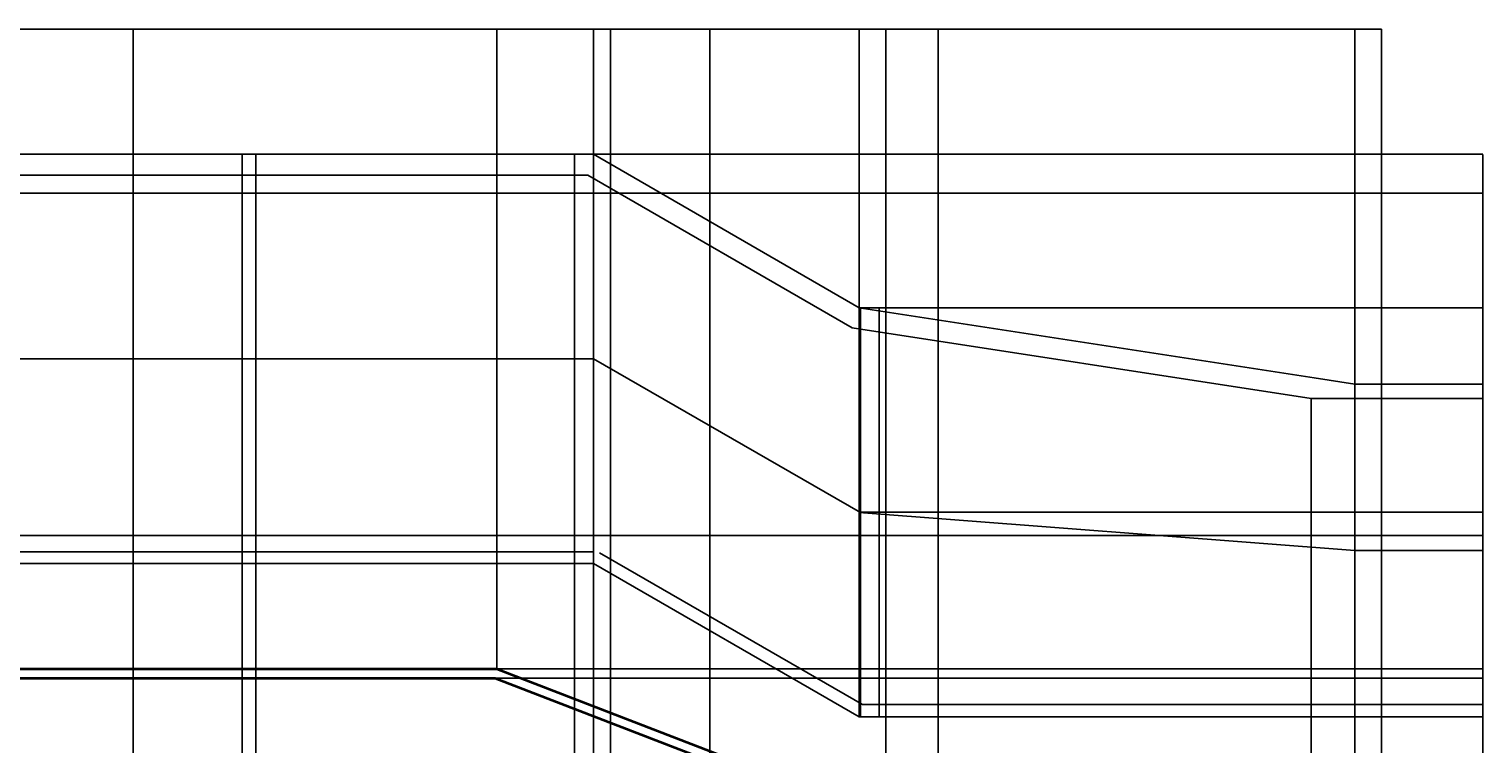
# Model space of a CAD drawing. Units: millimetres. Extents: x 2845 to 7170, y 3531 to 6858.
# Tile 3 of 3: x 4328 to 7170, y 5460 to 6858. Entities that reach past the tile are written whole.
import ezdxf

# ---------------------------------------------------------------- set-up
doc = ezdxf.new("R2010")
doc.units = ezdxf.units.MM
for name, color, linetype, lineweight in [('A-ANNO-DIMS', 2, 'Continuous', 18), ('A-FURN-CTOP', 6, 'Continuous', 35), ('A-FURN-UPPR', 4, 'Continuous', 25)]:
    doc.layers.add(name, color=color, linetype=linetype, lineweight=lineweight)
doc.styles.get("Standard").update_dxf_attribs({"font": 'arial.ttf'})
doc.dimstyles.get("Standard").update_dxf_attribs({"dimtxt": 0.18, "dimasz": 0.18, "dimexe": 0.18, "dimexo": 0.0625, "dimgap": 0.09, "dimtad": 0, "dimtih": 1, "dimtoh": 1, "dimdec": 4, "dimzin": 0, "dimdsep": 46, "dimtxsty": 'Standard', "dimcen": 0.09, "dimadec": 0, "dimazin": 0, "dimtfac": 1, "dimtdec": 4, "dimtofl": 0, "dimtmove": 0, "dimatfit": 3, "dimfxl": 1, "dimtolj": 1, "dimtzin": 0, "dimarcsym": 0})

# ---------------------------------------------------------------- blocks, each defined once
blk = doc.blocks.new('*D1')
at = {"layer": 'A-ANNO-DIMS', "color": 0, "lineweight": -2, "transparency": 16777216}
for p, q in [((3042.6, 6659.7), (2844.7, 6659.7)), ((2844.9, 6659.5), (2844.9, 5194.4)), ((2844.9, 3728.9), (2844.9, 5194)), ((6608, 3728.7), (2844.7, 3728.7))]:
    blk.add_line(p, q, dxfattribs=at)
at = {"layer": 'A-ANNO-DIMS', "color": 0, "transparency": 16777216}
for points in [[(2844.9, 6659.5), (2844.9, 6659.5), (2844.9, 6659.7)], [(2844.9, 3728.9), (2844.9, 3728.9), (2844.9, 3728.7)]]:
    blk.add_solid(points, dxfattribs=at)
at = {"layer": 'Defpoints', "color": 0, "transparency": 16777216}
for p in [(2844.9, 6659.7), (3042.7, 6659.7), (6608.1, 3728.7)]:
    blk.add_point(p, dxfattribs=at)
at = {"layer": 'A-ANNO-DIMS', "color": 0, "transparency": 16777216, "insert": (2844.9, 5194.2), "char_height": 0.18, "attachment_point": 5}
blk.add_mtext('\\A1;2931', dxfattribs=at)
blk = doc.blocks.new('*D2')
at = {"layer": 'A-ANNO-DIMS', "color": 0, "lineweight": -2, "transparency": 16777216}
for p, q in [((3042.7, 6659.8), (3042.7, 6857.7)), ((3042.8, 6857.5), (5006.9, 6857.5)), ((6971.9, 6857.5), (5007.8, 6857.5)), ((6972.1, 4944.1), (6972.1, 6857.7))]:
    blk.add_line(p, q, dxfattribs=at)
at = {"layer": 'A-ANNO-DIMS', "color": 0, "transparency": 16777216}
for points in [[(3042.8, 6857.5), (3042.8, 6857.4), (3042.7, 6857.5)], [(6971.9, 6857.5), (6971.9, 6857.4), (6972.1, 6857.5)]]:
    blk.add_solid(points, dxfattribs=at)
at = {"layer": 'Defpoints', "color": 0, "transparency": 16777216}
for p in [(6972.1, 6857.5), (3042.7, 6659.7), (6972.1, 4944.1)]:
    blk.add_point(p, dxfattribs=at)
at = {"layer": 'A-ANNO-DIMS', "color": 0, "transparency": 16777216, "insert": (5007.4, 6857.5), "char_height": 0.18, "attachment_point": 5}
blk.add_mtext('\\A1;3929.4', dxfattribs=at)
blk = doc.blocks.new('*D6')
at = {"layer": 'A-ANNO-DIMS', "color": 0, "lineweight": -2, "transparency": 16777216}
for p, q in [((4121.4, 6537), (4121.4, 6857.7)), ((4121.6, 6857.5), (4325.9, 6857.5)), ((4531.1, 6857.5), (4326.7, 6857.5)), ((4531.3, 6612.8), (4531.3, 6857.7))]:
    blk.add_line(p, q, dxfattribs=at)
at = {"layer": 'A-ANNO-DIMS', "color": 0, "transparency": 16777216}
for points in [[(4121.6, 6857.5), (4121.6, 6857.4), (4121.4, 6857.5)], [(4531.1, 6857.5), (4531.1, 6857.4), (4531.3, 6857.5)]]:
    blk.add_solid(points, dxfattribs=at)
at = {"layer": 'Defpoints', "color": 0, "transparency": 16777216}
for p in [(4531.3, 6857.5), (4531.3, 6612.8), (4121.4, 6537)]:
    blk.add_point(p, dxfattribs=at)
at = {"layer": 'A-ANNO-DIMS', "color": 0, "transparency": 16777216, "insert": (4326.3, 6857.5), "char_height": 0.18, "attachment_point": 5}
blk.add_mtext('\\A1;409.9', dxfattribs=at)
blk = doc.blocks.new('*D7')
at = {"layer": 'A-ANNO-DIMS', "color": 0, "lineweight": -2, "transparency": 16777216}
for p, q in [((4531.3, 6612.8), (4531.3, 6857.7)), ((4531.4, 6857.5), (4981, 6857.5)), ((5431.1, 6857.5), (4981.6, 6857.5)), ((5431.3, 6612.8), (5431.3, 6857.7))]:
    blk.add_line(p, q, dxfattribs=at)
at = {"layer": 'A-ANNO-DIMS', "color": 0, "transparency": 16777216}
for points in [[(4531.4, 6857.5), (4531.4, 6857.4), (4531.3, 6857.5)], [(5431.1, 6857.5), (5431.1, 6857.4), (5431.3, 6857.5)]]:
    blk.add_solid(points, dxfattribs=at)
at = {"layer": 'Defpoints', "color": 0, "transparency": 16777216}
for p in [(5431.3, 6857.5), (4531.3, 6612.8), (5431.3, 6612.8)]:
    blk.add_point(p, dxfattribs=at)
at = {"layer": 'A-ANNO-DIMS', "color": 0, "transparency": 16777216, "insert": (4981.3, 6857.5), "char_height": 0.18, "attachment_point": 5}
blk.add_mtext('\\A1;900', dxfattribs=at)
blk = doc.blocks.new('*D8')
at = {"layer": 'A-ANNO-DIMS', "color": 0, "lineweight": -2, "transparency": 16777216}
for p, q in [((5431.3, 6612.8), (5431.3, 6857.7)), ((5431.4, 6857.5), (5690.7, 6857.5)), ((5950.7, 6857.5), (5691.5, 6857.5)), ((5950.9, 6312.8), (5950.9, 6857.7))]:
    blk.add_line(p, q, dxfattribs=at)
at = {"layer": 'A-ANNO-DIMS', "color": 0, "transparency": 16777216}
for points in [[(5431.4, 6857.5), (5431.4, 6857.4), (5431.3, 6857.5)], [(5950.7, 6857.5), (5950.7, 6857.4), (5950.9, 6857.5)]]:
    blk.add_solid(points, dxfattribs=at)
at = {"layer": 'Defpoints', "color": 0, "transparency": 16777216}
for p in [(5950.9, 6857.5), (5431.3, 6612.8), (5950.9, 6312.8)]:
    blk.add_point(p, dxfattribs=at)
at = {"layer": 'A-ANNO-DIMS', "color": 0, "transparency": 16777216, "insert": (5691.1, 6857.5), "char_height": 0.18, "attachment_point": 5}
blk.add_mtext('\\A1;519.6', dxfattribs=at)
blk = doc.blocks.new('*D9')
at = {"layer": 'A-ANNO-DIMS', "color": 0, "lineweight": -2, "transparency": 16777216}
for p, q in [((5950.9, 6312.8), (5950.9, 6857.7)), ((5951.1, 6857.5), (6435.1, 6857.5)), ((6919.6, 6857.5), (6435.6, 6857.5)), ((6919.8, 6163.6), (6919.8, 6857.7))]:
    blk.add_line(p, q, dxfattribs=at)
at = {"layer": 'A-ANNO-DIMS', "color": 0, "transparency": 16777216}
for points in [[(5951.1, 6857.5), (5951.1, 6857.4), (5950.9, 6857.5)], [(6919.6, 6857.5), (6919.6, 6857.4), (6919.8, 6857.5)]]:
    blk.add_solid(points, dxfattribs=at)
at = {"layer": 'Defpoints', "color": 0, "transparency": 16777216}
for p in [(6919.8, 6857.5), (5950.9, 6312.8), (6919.8, 6163.5)]:
    blk.add_point(p, dxfattribs=at)
at = {"layer": 'A-ANNO-DIMS', "color": 0, "transparency": 16777216, "insert": (6435.4, 6857.5), "char_height": 0.18, "attachment_point": 5}
blk.add_mtext('\\A1;969', dxfattribs=at)
blk = doc.blocks.new('*D23')
at = {"layer": 'A-ANNO-DIMS', "color": 0, "lineweight": -2, "transparency": 16777216}
for p, q in [((4121.5, 6537), (7170, 6537)), ((7169.8, 6536.8), (7169.8, 6202.3)), ((7169.8, 5867.4), (7169.8, 6201.9)), ((4121.5, 5867.2), (7170, 5867.2))]:
    blk.add_line(p, q, dxfattribs=at)
at = {"layer": 'A-ANNO-DIMS', "color": 0, "transparency": 16777216}
for points in [[(7169.8, 6536.8), (7169.8, 6536.8), (7169.8, 6537)], [(7169.8, 5867.4), (7169.8, 5867.4), (7169.8, 5867.2)]]:
    blk.add_solid(points, dxfattribs=at)
at = {"layer": 'Defpoints', "color": 0, "transparency": 16777216}
for p in [(4121.4, 6537), (7169.8, 6537), (4121.4, 5867.2)]:
    blk.add_point(p, dxfattribs=at)
at = {"layer": 'A-ANNO-DIMS', "color": 0, "transparency": 16777216, "insert": (7169.8, 6202.1), "char_height": 0.18, "attachment_point": 5}
blk.add_mtext('\\A1;669.7', dxfattribs=at)
blk = doc.blocks.new('*D24')
at = {"layer": 'A-ANNO-DIMS', "color": 0, "lineweight": -2, "transparency": 16777216}
for p, q in [((3939, 6612.8), (7170, 6612.8)), ((7169.8, 6612.6), (7169.8, 6575.1)), ((7169.8, 6537.2), (7169.8, 6574.7)), ((4121.5, 6537), (7170, 6537))]:
    blk.add_line(p, q, dxfattribs=at)
at = {"layer": 'A-ANNO-DIMS', "color": 0, "transparency": 16777216}
for points in [[(7169.8, 6612.6), (7169.8, 6612.6), (7169.8, 6612.8)], [(7169.8, 6537.2), (7169.8, 6537.2), (7169.8, 6537)]]:
    blk.add_solid(points, dxfattribs=at)
at = {"layer": 'Defpoints', "color": 0, "transparency": 16777216}
for p in [(3939, 6612.8), (7169.8, 6612.8), (4121.4, 6537)]:
    blk.add_point(p, dxfattribs=at)
at = {"layer": 'A-ANNO-DIMS', "color": 0, "transparency": 16777216, "insert": (7169.8, 6574.9), "char_height": 0.18, "attachment_point": 5}
blk.add_mtext('\\A1;75.77', dxfattribs=at)
blk = doc.blocks.new('*D25')
at = {"layer": 'A-ANNO-DIMS', "color": 0, "lineweight": -2, "transparency": 16777216}
for p, q in [((4531.2, 5835.4), (2844.7, 5835.4)), ((2844.9, 5835.2), (2844.9, 5824.2)), ((4531.2, 5812.8), (2844.7, 5812.8)), ((2844.9, 5812.9), (2844.9, 5823.9))]:
    blk.add_line(p, q, dxfattribs=at)
at = {"layer": 'A-ANNO-DIMS', "color": 0, "transparency": 16777216}
for points in [[(2844.9, 5835.2), (2844.9, 5835.2), (2844.9, 5835.4)], [(2844.9, 5812.9), (2844.9, 5812.9), (2844.9, 5812.8)]]:
    blk.add_solid(points, dxfattribs=at)
at = {"layer": 'Defpoints', "color": 0, "transparency": 16777216}
for p in [(2844.9, 5835.4), (4531.3, 5835.4), (4531.3, 5812.8)]:
    blk.add_point(p, dxfattribs=at)
at = {"layer": 'A-ANNO-DIMS', "color": 0, "transparency": 16777216, "insert": (2844.9, 5824.1), "char_height": 0.18, "attachment_point": 5}
blk.add_mtext('\\A1;22.6', dxfattribs=at)
blk = doc.blocks.new('*D26')
at = {"layer": 'A-ANNO-DIMS', "color": 0, "lineweight": -2, "transparency": 16777216}
for p, q in [((4744.4, 6212.8), (2844.7, 6212.8)), ((2844.9, 6212.6), (2844.9, 6024.2)), ((2844.9, 5835.5), (2844.9, 6023.9)), ((4531.2, 5835.4), (2844.7, 5835.4))]:
    blk.add_line(p, q, dxfattribs=at)
at = {"layer": 'A-ANNO-DIMS', "color": 0, "transparency": 16777216}
for points in [[(2844.9, 6212.6), (2844.9, 6212.6), (2844.9, 6212.8)], [(2844.9, 5835.5), (2844.9, 5835.5), (2844.9, 5835.4)]]:
    blk.add_solid(points, dxfattribs=at)
at = {"layer": 'Defpoints', "color": 0, "transparency": 16777216}
for p in [(2844.9, 6212.8), (4744.4, 6212.8), (4531.3, 5835.4)]:
    blk.add_point(p, dxfattribs=at)
at = {"layer": 'A-ANNO-DIMS', "color": 0, "transparency": 16777216, "insert": (2844.9, 6024.1), "char_height": 0.18, "attachment_point": 5}
blk.add_mtext('\\A1;377.4', dxfattribs=at)
blk = doc.blocks.new('*D27')
at = {"layer": 'A-ANNO-DIMS', "color": 0, "lineweight": -2, "transparency": 16777216}
for p, q in [((4531.2, 6571.7), (2844.7, 6571.7)), ((2844.9, 6571.6), (2844.9, 6392.4)), ((2844.9, 6212.9), (2844.9, 6392.1)), ((4744.4, 6212.8), (2844.7, 6212.8))]:
    blk.add_line(p, q, dxfattribs=at)
at = {"layer": 'A-ANNO-DIMS', "color": 0, "transparency": 16777216}
for points in [[(2844.9, 6571.6), (2844.9, 6571.6), (2844.9, 6571.7)], [(2844.9, 6212.9), (2844.9, 6212.9), (2844.9, 6212.8)]]:
    blk.add_solid(points, dxfattribs=at)
at = {"layer": 'Defpoints', "color": 0, "transparency": 16777216}
for p in [(2844.9, 6571.7), (4531.3, 6571.7), (4744.4, 6212.8)]:
    blk.add_point(p, dxfattribs=at)
at = {"layer": 'A-ANNO-DIMS', "color": 0, "transparency": 16777216, "insert": (2844.9, 6392.2), "char_height": 0.18, "attachment_point": 5}
blk.add_mtext('\\A1;359', dxfattribs=at)
blk = doc.blocks.new('*D28')
at = {"layer": 'A-ANNO-DIMS', "color": 0, "lineweight": -2, "transparency": 16777216}
for p, q in [((4531.2, 6612.8), (2844.7, 6612.8)), ((2844.9, 6612.6), (2844.9, 6592.4)), ((4531.2, 6571.7), (2844.7, 6571.7)), ((2844.9, 6571.9), (2844.9, 6592.1))]:
    blk.add_line(p, q, dxfattribs=at)
at = {"layer": 'A-ANNO-DIMS', "color": 0, "transparency": 16777216}
for points in [[(2844.9, 6612.6), (2844.9, 6612.6), (2844.9, 6612.8)], [(2844.9, 6571.9), (2844.9, 6571.9), (2844.9, 6571.7)]]:
    blk.add_solid(points, dxfattribs=at)
at = {"layer": 'Defpoints', "color": 0, "transparency": 16777216}
for p in [(2844.9, 6612.8), (4531.3, 6612.8), (4531.3, 6571.7)]:
    blk.add_point(p, dxfattribs=at)
at = {"layer": 'A-ANNO-DIMS', "color": 0, "transparency": 16777216, "insert": (2844.9, 6592.2), "char_height": 0.18, "attachment_point": 5}
blk.add_mtext('\\A1;41.03', dxfattribs=at)
blk = doc.blocks.new('*D29')
at = {"layer": 'A-ANNO-DIMS', "color": 0, "lineweight": -2, "transparency": 16777216}
for p, q in [((4531.3, 5812.7), (4531.3, 3530.8)), ((4744.4, 5812.7), (4744.4, 3530.8)), ((4531.4, 3531), (4637.4, 3531)), ((4744.3, 3531), (4638.3, 3531))]:
    blk.add_line(p, q, dxfattribs=at)
at = {"layer": 'A-ANNO-DIMS', "color": 0, "transparency": 16777216}
for points in [[(4531.4, 3531), (4531.4, 3530.9), (4531.3, 3531)], [(4744.3, 3531), (4744.3, 3530.9), (4744.4, 3531)]]:
    blk.add_solid(points, dxfattribs=at)
at = {"layer": 'Defpoints', "color": 0, "transparency": 16777216}
for p in [(4531.3, 5812.8), (4744.4, 5812.8), (4744.4, 3531)]:
    blk.add_point(p, dxfattribs=at)
at = {"layer": 'A-ANNO-DIMS', "color": 0, "transparency": 16777216, "insert": (4637.9, 3531), "char_height": 0.18, "attachment_point": 5}
blk.add_mtext('\\A1;213.17', dxfattribs=at)
blk = doc.blocks.new('*D30')
at = {"layer": 'A-ANNO-DIMS', "color": 0, "lineweight": -2, "transparency": 16777216}
for p, q in [((4744.4, 5812.7), (4744.4, 3530.8)), ((4771.2, 5812.7), (4771.2, 3530.8)), ((4744.6, 3531), (4757.4, 3531)), ((4771, 3531), (4758.3, 3531))]:
    blk.add_line(p, q, dxfattribs=at)
at = {"layer": 'A-ANNO-DIMS', "color": 0, "transparency": 16777216}
for points in [[(4744.6, 3531), (4744.6, 3530.9), (4744.4, 3531)], [(4771, 3531), (4771, 3530.9), (4771.2, 3531)]]:
    blk.add_solid(points, dxfattribs=at)
at = {"layer": 'Defpoints', "color": 0, "transparency": 16777216}
for p in [(4744.4, 5812.8), (4771.2, 5812.8), (4771.2, 3531)]:
    blk.add_point(p, dxfattribs=at)
at = {"layer": 'A-ANNO-DIMS', "color": 0, "transparency": 16777216, "insert": (4757.8, 3531), "char_height": 0.18, "attachment_point": 5}
blk.add_mtext('\\A1;26.776', dxfattribs=at)
blk = doc.blocks.new('*D31')
at = {"layer": 'A-ANNO-DIMS', "color": 0, "lineweight": -2, "transparency": 16777216}
for p, q in [((5394.2, 5812.7), (5394.2, 3530.8)), ((5431.3, 5812.7), (5431.3, 3530.8)), ((5394.4, 3531), (5412.3, 3531)), ((5431.1, 3531), (5413.1, 3531))]:
    blk.add_line(p, q, dxfattribs=at)
at = {"layer": 'A-ANNO-DIMS', "color": 0, "transparency": 16777216}
for points in [[(5394.4, 3531), (5394.4, 3530.9), (5394.2, 3531)], [(5431.1, 3531), (5431.1, 3530.9), (5431.3, 3531)]]:
    blk.add_solid(points, dxfattribs=at)
at = {"layer": 'Defpoints', "color": 0, "transparency": 16777216}
for p in [(5394.2, 5812.8), (5431.3, 5812.8), (5431.3, 3531)]:
    blk.add_point(p, dxfattribs=at)
at = {"layer": 'A-ANNO-DIMS', "color": 0, "transparency": 16777216, "insert": (5412.7, 3531), "char_height": 0.18, "attachment_point": 5}
blk.add_mtext('\\A1;37.06', dxfattribs=at)
blk = doc.blocks.new('*D32')
at = {"layer": 'A-ANNO-DIMS', "color": 0, "lineweight": -2, "transparency": 16777216}
for p, q in [((5431.3, 6612.8), (7170, 6612.8)), ((7169.8, 6612.6), (7169.8, 6462.9)), ((7169.8, 6312.9), (7169.8, 6462.6)), ((5950.9, 6312.8), (7170, 6312.8))]:
    blk.add_line(p, q, dxfattribs=at)
at = {"layer": 'A-ANNO-DIMS', "color": 0, "transparency": 16777216}
for points in [[(7169.8, 6612.6), (7169.8, 6612.6), (7169.8, 6612.8)], [(7169.8, 6312.9), (7169.8, 6312.9), (7169.8, 6312.8)]]:
    blk.add_solid(points, dxfattribs=at)
at = {"layer": 'Defpoints', "color": 0, "transparency": 16777216}
for p in [(5431.3, 6612.8), (5950.9, 6312.8), (7169.8, 6312.8)]:
    blk.add_point(p, dxfattribs=at)
at = {"layer": 'A-ANNO-DIMS', "color": 0, "transparency": 16777216, "insert": (7169.8, 6462.8), "char_height": 0.18, "attachment_point": 5}
blk.add_mtext('\\A1;300', dxfattribs=at)
blk = doc.blocks.new('*D33')
at = {"layer": 'A-ANNO-DIMS', "color": 0, "lineweight": -2, "transparency": 16777216}
for p, q in [((6919.9, 5537.2), (7170, 5537.2)), ((7169.8, 5537), (7169.8, 5525.1)), ((7169.8, 5512.9), (7169.8, 5524.8)), ((6919.9, 5512.8), (7170, 5512.8))]:
    blk.add_line(p, q, dxfattribs=at)
at = {"layer": 'A-ANNO-DIMS', "color": 0, "transparency": 16777216}
for points in [[(7169.8, 5537), (7169.8, 5537), (7169.8, 5537.2)], [(7169.8, 5512.9), (7169.8, 5512.9), (7169.8, 5512.8)]]:
    blk.add_solid(points, dxfattribs=at)
at = {"layer": 'Defpoints', "color": 0, "transparency": 16777216}
for p in [(6919.8, 5537.2), (7169.8, 5537.2), (6919.8, 5512.8)]:
    blk.add_point(p, dxfattribs=at)
at = {"layer": 'A-ANNO-DIMS', "color": 0, "transparency": 16777216, "insert": (7169.8, 5525), "char_height": 0.18, "attachment_point": 5}
blk.add_mtext('\\A1;24.414', dxfattribs=at)
blk = doc.blocks.new('*D34')
at = {"layer": 'A-ANNO-DIMS', "color": 0, "lineweight": -2, "transparency": 16777216}
for p, q in [((6919.9, 5838.1), (7170, 5838.1)), ((7169.8, 5837.9), (7169.8, 5687.8)), ((7169.8, 5537.4), (7169.8, 5687.5)), ((6919.9, 5537.2), (7170, 5537.2))]:
    blk.add_line(p, q, dxfattribs=at)
at = {"layer": 'A-ANNO-DIMS', "color": 0, "transparency": 16777216}
for points in [[(7169.8, 5837.9), (7169.8, 5837.9), (7169.8, 5838.1)], [(7169.8, 5537.4), (7169.8, 5537.4), (7169.8, 5537.2)]]:
    blk.add_solid(points, dxfattribs=at)
at = {"layer": 'Defpoints', "color": 0, "transparency": 16777216}
for p in [(6919.8, 5838.1), (7169.8, 5838.1), (6919.8, 5537.2)]:
    blk.add_point(p, dxfattribs=at)
at = {"layer": 'A-ANNO-DIMS', "color": 0, "transparency": 16777216, "insert": (7169.8, 5687.7), "char_height": 0.18, "attachment_point": 5}
blk.add_mtext('\\A1;300.96', dxfattribs=at)
blk = doc.blocks.new('*D35')
at = {"layer": 'A-ANNO-DIMS', "color": 0, "lineweight": -2, "transparency": 16777216}
for p, q in [((6919.9, 6135.2), (7170, 6135.2)), ((7169.8, 6135), (7169.8, 5986.8)), ((7169.8, 5838.3), (7169.8, 5986.5)), ((6919.9, 5838.1), (7170, 5838.1))]:
    blk.add_line(p, q, dxfattribs=at)
at = {"layer": 'A-ANNO-DIMS', "color": 0, "transparency": 16777216}
for points in [[(7169.8, 6135), (7169.8, 6135), (7169.8, 6135.2)], [(7169.8, 5838.3), (7169.8, 5838.3), (7169.8, 5838.1)]]:
    blk.add_solid(points, dxfattribs=at)
at = {"layer": 'Defpoints', "color": 0, "transparency": 16777216}
for p in [(6919.8, 6135.2), (7169.8, 6135.2), (6919.8, 5838.1)]:
    blk.add_point(p, dxfattribs=at)
at = {"layer": 'A-ANNO-DIMS', "color": 0, "transparency": 16777216, "insert": (7169.8, 5986.7), "char_height": 0.18, "attachment_point": 5}
blk.add_mtext('\\A1;297.06', dxfattribs=at)
blk = doc.blocks.new('*D36')
at = {"layer": 'A-ANNO-DIMS', "color": 0, "lineweight": -2, "transparency": 16777216}
for p, q in [((6919.9, 6163.5), (7170, 6163.5)), ((7169.8, 6163.3), (7169.8, 6149.5)), ((7169.8, 6135.4), (7169.8, 6149.2)), ((6919.9, 6135.2), (7170, 6135.2))]:
    blk.add_line(p, q, dxfattribs=at)
at = {"layer": 'A-ANNO-DIMS', "color": 0, "transparency": 16777216}
for points in [[(7169.8, 6163.3), (7169.8, 6163.3), (7169.8, 6163.5)], [(7169.8, 6135.4), (7169.8, 6135.4), (7169.8, 6135.2)]]:
    blk.add_solid(points, dxfattribs=at)
at = {"layer": 'Defpoints', "color": 0, "transparency": 16777216}
for p in [(6919.8, 6163.5), (7169.8, 6163.5), (6919.8, 6135.2)]:
    blk.add_point(p, dxfattribs=at)
at = {"layer": 'A-ANNO-DIMS', "color": 0, "transparency": 16777216, "insert": (7169.8, 6149.3), "char_height": 0.18, "attachment_point": 5}
blk.add_mtext('\\A1;28.314', dxfattribs=at)
blk = doc.blocks.new('*D37')
at = {"layer": 'A-ANNO-DIMS', "color": 0, "lineweight": -2, "transparency": 16777216}
for p, q in [((5950.9, 5912.8), (7170, 5912.8)), ((7169.8, 5912.6), (7169.8, 5712.9)), ((7169.8, 5512.9), (7169.8, 5712.6)), ((5950.9, 5512.8), (7170, 5512.8))]:
    blk.add_line(p, q, dxfattribs=at)
at = {"layer": 'A-ANNO-DIMS', "color": 0, "transparency": 16777216}
for points in [[(7169.8, 5912.6), (7169.8, 5912.6), (7169.8, 5912.8)], [(7169.8, 5512.9), (7169.8, 5512.9), (7169.8, 5512.8)]]:
    blk.add_solid(points, dxfattribs=at)
at = {"layer": 'Defpoints', "color": 0, "transparency": 16777216}
for p in [(5950.9, 5912.8), (7169.8, 5912.8), (5950.9, 5512.8)]:
    blk.add_point(p, dxfattribs=at)
at = {"layer": 'A-ANNO-DIMS', "color": 0, "transparency": 16777216, "insert": (7169.8, 5712.8), "char_height": 0.18, "attachment_point": 5}
blk.add_mtext('\\A1;400', dxfattribs=at)
blk = doc.blocks.new('*D38')
at = {"layer": 'A-ANNO-DIMS', "color": 0, "lineweight": -2, "transparency": 16777216}
for p, q in [((5950.9, 6312.8), (7170, 6312.8)), ((7169.8, 6312.6), (7169.8, 6112.9)), ((7169.8, 5912.9), (7169.8, 6112.6)), ((5950.9, 5912.8), (7170, 5912.8))]:
    blk.add_line(p, q, dxfattribs=at)
at = {"layer": 'A-ANNO-DIMS', "color": 0, "transparency": 16777216}
for points in [[(7169.8, 6312.6), (7169.8, 6312.6), (7169.8, 6312.8)], [(7169.8, 5912.9), (7169.8, 5912.9), (7169.8, 5912.8)]]:
    blk.add_solid(points, dxfattribs=at)
at = {"layer": 'Defpoints', "color": 0, "transparency": 16777216}
for p in [(5950.9, 6312.8), (7169.8, 6312.8), (5950.9, 5912.8)]:
    blk.add_point(p, dxfattribs=at)
at = {"layer": 'A-ANNO-DIMS', "color": 0, "transparency": 16777216, "insert": (7169.8, 6112.8), "char_height": 0.18, "attachment_point": 5}
blk.add_mtext('\\A1;400', dxfattribs=at)
blk = doc.blocks.new('*D39')
at = {"layer": 'A-ANNO-DIMS', "color": 0, "lineweight": -2, "transparency": 16777216}
for p, q in [((6834.1, 6135.1), (6834.1, 3530.8)), ((6919.8, 6135.1), (6919.8, 3530.8)), ((6834.3, 3531), (6876.6, 3531)), ((6919.6, 3531), (6877.4, 3531))]:
    blk.add_line(p, q, dxfattribs=at)
at = {"layer": 'A-ANNO-DIMS', "color": 0, "transparency": 16777216}
for points in [[(6834.3, 3531), (6834.3, 3530.9), (6834.1, 3531)], [(6919.6, 3531), (6919.6, 3530.9), (6919.8, 3531)]]:
    blk.add_solid(points, dxfattribs=at)
at = {"layer": 'Defpoints', "color": 0, "transparency": 16777216}
for p in [(6834.1, 6135.2), (6919.8, 6135.2), (6919.8, 3531)]:
    blk.add_point(p, dxfattribs=at)
at = {"layer": 'A-ANNO-DIMS', "color": 0, "transparency": 16777216, "insert": (6877, 3531), "char_height": 0.18, "attachment_point": 5}
blk.add_mtext('\\A1;85.67', dxfattribs=at)
blk = doc.blocks.new('*D41')
at = {"layer": 'A-ANNO-DIMS', "color": 0, "lineweight": -2, "transparency": 16777216}
for p, q in [((3939, 5588.8), (7170, 5588.8)), ((7169.8, 5588.6), (7169.8, 5439.4)), ((7169.8, 5289.7), (7169.8, 5439)), ((3939, 5289.6), (7170, 5289.6))]:
    blk.add_line(p, q, dxfattribs=at)
at = {"layer": 'A-ANNO-DIMS', "color": 0, "transparency": 16777216}
for points in [[(7169.8, 5588.6), (7169.8, 5588.6), (7169.8, 5588.8)], [(7169.8, 5289.7), (7169.8, 5289.7), (7169.8, 5289.6)]]:
    blk.add_solid(points, dxfattribs=at)
at = {"layer": 'Defpoints', "color": 0, "transparency": 16777216}
for p in [(3939, 5588.8), (7169.8, 5588.8), (3939, 5289.6)]:
    blk.add_point(p, dxfattribs=at)
at = {"layer": 'A-ANNO-DIMS', "color": 0, "transparency": 16777216, "insert": (7169.8, 5439.2), "char_height": 0.18, "attachment_point": 5}
blk.add_mtext('\\A1;299.2', dxfattribs=at)
blk = doc.blocks.new('*D42')
at = {"layer": 'A-ANNO-DIMS', "color": 0, "lineweight": -2, "transparency": 16777216}
for p, q in [((3939, 5606.6), (7170, 5606.6)), ((7169.8, 5606.5), (7169.8, 5597.9)), ((3939, 5588.8), (7170, 5588.8)), ((7169.8, 5589), (7169.8, 5597.5))]:
    blk.add_line(p, q, dxfattribs=at)
at = {"layer": 'A-ANNO-DIMS', "color": 0, "transparency": 16777216}
for points in [[(7169.8, 5606.5), (7169.8, 5606.5), (7169.8, 5606.6)], [(7169.8, 5589), (7169.8, 5589), (7169.8, 5588.8)]]:
    blk.add_solid(points, dxfattribs=at)
at = {"layer": 'Defpoints', "color": 0, "transparency": 16777216}
for p in [(3939, 5606.6), (7169.8, 5606.6), (3939, 5588.8)]:
    blk.add_point(p, dxfattribs=at)
at = {"layer": 'A-ANNO-DIMS', "color": 0, "transparency": 16777216, "insert": (7169.8, 5597.7), "char_height": 0.18, "attachment_point": 5}
blk.add_mtext('\\A1;17.853', dxfattribs=at)
blk = doc.blocks.new('*D43')
at = {"layer": 'A-ANNO-DIMS', "color": 0, "lineweight": -2, "transparency": 16777216}
for p, q in [((3939, 5606.7), (3939, 6857.7)), ((3939.1, 6857.5), (4590.2, 6857.5)), ((5242.1, 6857.5), (4591.1, 6857.5)), ((5242.3, 5606.7), (5242.3, 6857.7))]:
    blk.add_line(p, q, dxfattribs=at)
at = {"layer": 'A-ANNO-DIMS', "color": 0, "transparency": 16777216}
for points in [[(3939.1, 6857.5), (3939.1, 6857.4), (3939, 6857.5)], [(5242.1, 6857.5), (5242.1, 6857.4), (5242.3, 6857.5)]]:
    blk.add_solid(points, dxfattribs=at)
at = {"layer": 'Defpoints', "color": 0, "transparency": 16777216}
for p in [(5242.3, 6857.5), (3939, 5606.6), (5242.3, 5606.6)]:
    blk.add_point(p, dxfattribs=at)
at = {"layer": 'A-ANNO-DIMS', "color": 0, "transparency": 16777216, "insert": (4590.6, 6857.5), "char_height": 0.18, "attachment_point": 5}
blk.add_mtext('\\A1;1303.3', dxfattribs=at)
blk = doc.blocks.new('*D44')
at = {"layer": 'A-ANNO-DIMS', "color": 0, "lineweight": -2, "transparency": 16777216}
for p, q in [((3939, 5289.6), (3939, 6857.7)), ((3939.1, 6857.5), (4701.3, 6857.5)), ((5464.4, 6857.5), (4702.2, 6857.5)), ((5464.6, 5289.6), (5464.6, 6857.7))]:
    blk.add_line(p, q, dxfattribs=at)
at = {"layer": 'A-ANNO-DIMS', "color": 0, "transparency": 16777216}
for points in [[(3939.1, 6857.5), (3939.1, 6857.4), (3939, 6857.5)], [(5464.4, 6857.5), (5464.4, 6857.4), (5464.6, 6857.5)]]:
    blk.add_solid(points, dxfattribs=at)
at = {"layer": 'Defpoints', "color": 0, "transparency": 16777216}
for p in [(5464.6, 6857.5), (3939, 5289.6), (5464.6, 5289.6)]:
    blk.add_point(p, dxfattribs=at)
at = {"layer": 'A-ANNO-DIMS', "color": 0, "transparency": 16777216, "insert": (4701.8, 6857.5), "char_height": 0.18, "attachment_point": 5}
blk.add_mtext('\\A1;1525.6', dxfattribs=at)
blk = doc.blocks.new('*D45')
at = {"layer": 'A-ANNO-DIMS', "color": 0, "lineweight": -2, "transparency": 16777216}
for p, q in [((5464.6, 5289.6), (5464.6, 6857.7)), ((5464.8, 6857.5), (5561.2, 6857.5)), ((5658.6, 6857.5), (5562.1, 6857.5)), ((5658.7, 5426.7), (5658.7, 6857.7))]:
    blk.add_line(p, q, dxfattribs=at)
at = {"layer": 'A-ANNO-DIMS', "color": 0, "transparency": 16777216}
for points in [[(5464.8, 6857.5), (5464.8, 6857.4), (5464.6, 6857.5)], [(5658.6, 6857.5), (5658.6, 6857.4), (5658.7, 6857.5)]]:
    blk.add_solid(points, dxfattribs=at)
at = {"layer": 'Defpoints', "color": 0, "transparency": 16777216}
for p in [(5658.7, 6857.5), (5658.7, 5426.7), (5464.6, 5289.6)]:
    blk.add_point(p, dxfattribs=at)
at = {"layer": 'A-ANNO-DIMS', "color": 0, "transparency": 16777216, "insert": (5561.7, 6857.5), "char_height": 0.18, "attachment_point": 5}
blk.add_mtext('\\A1;194.16', dxfattribs=at)
blk = doc.blocks.new('*D69')
at = {"layer": 'A-ANNO-DIMS', "color": 0, "lineweight": -2, "transparency": 16777216}
for p, q in [((6003, 5004.7), (6003, 6857.7)), ((6003.2, 6857.5), (6053.8, 6857.5)), ((6105.3, 6857.5), (6054.7, 6857.5)), ((6105.5, 5039.1), (6105.5, 6857.7))]:
    blk.add_line(p, q, dxfattribs=at)
at = {"layer": 'A-ANNO-DIMS', "color": 0, "transparency": 16777216}
for points in [[(6003.2, 6857.5), (6003.2, 6857.4), (6003, 6857.5)], [(6105.3, 6857.5), (6105.3, 6857.4), (6105.5, 6857.5)]]:
    blk.add_solid(points, dxfattribs=at)
at = {"layer": 'Defpoints', "color": 0, "transparency": 16777216}
for p in [(6105.5, 6857.5), (6105.5, 5039), (6003, 5004.6)]:
    blk.add_point(p, dxfattribs=at)
at = {"layer": 'A-ANNO-DIMS', "color": 0, "transparency": 16777216, "insert": (6054.2, 6857.5), "char_height": 0.18, "attachment_point": 5}
blk.add_mtext('\\A1;102.43', dxfattribs=at)

msp = doc.modelspace()

# ---------------------------------------------------------------- linework, layer by layer
at = {"layer": 'A-FURN-CTOP', "extrusion": (0, 0, -1)}
for points in [[(-3938.9578, 5606.6435), (-5242.2853, 5606.6435), (-6084.9137, 5281.2335), (-6972.0668, 4944.0752), (-6607.6118, 4817.5346), (-5766.7252, 5156.141), (-5461.3127, 5271.7102), (-4164.5775, 5271.7102), (-3938.9578, 5271.7102)], [(-3938.9578, 5588.7906), (-5238.9578, 5588.7906), (-6078.5267, 5264.5621), (-6919.8193, 4944.8329), (-6608.0753, 4836.5939), (-5773.2194, 5172.7719), (-5464.5775, 5289.563), (-4164.5775, 5289.563), (-3938.9578, 5289.563)]]:
    msp.add_lwpolyline(points, dxfattribs=at)
at = {"layer": 'A-FURN-UPPR', "extrusion": (0, 0, -1)}
for p, q in [((4531.2682, 6612.7588), (4531.2682, 5812.7588)), ((4744.4359, 6612.7588), (4744.4359, 5812.7588)), ((4771.2123, 6612.7588), (4771.2123, 5812.7588)), ((5394.2056, 5812.7588), (5394.2056, 6612.7588)), ((5431.2682, 5812.7588), (5431.2682, 6612.7588)), ((5950.8834, 5512.7588), (5950.8834, 6312.7588)), ((5953.2342, 5512.7588), (5953.2342, 6312.7588)), ((5990.0362, 5512.7588), (5990.0362, 6312.7588)), ((4744.4359, 6212.7588), (5431.2682, 6212.7588)), ((5953.2342, 5912.7588), (5431.2682, 6212.7588)), ((6919.8193, 6163.4997), (6840.3914, 6175.7352)), ((6919.8193, 5512.7588), (6919.8193, 6163.4997)), ((5950.8834, 5912.7588), (6919.8193, 5838.1293)), ((4531.2682, 5835.359), (5431.2682, 5835.359)), ((4531.2682, 5812.7588), (5431.2682, 5812.7588))]:
    msp.add_line(p, q, dxfattribs=at)
for points in [[(-4531.2682, 6612.7588), (-5431.2682, 6612.7588), (-5950.8834, 6312.7588), (-6840.3914, 6175.7352)], [(-4531.2682, 6571.7311), (-5420.2748, 6571.7311), (-5937.0327, 6273.3808), (-6834.145, 6135.1857)], [(-6834.145, 6135.1857), (-6919.8193, 6135.1857)], [(-5443.4752, 5833.902), (-5957.4251, 5537.1728), (-6919.8193, 5537.1728)], [(-5431.2682, 5812.7588), (-5950.8834, 5512.7588), (-6919.8193, 5512.7588)]]:
    msp.add_lwpolyline(points, dxfattribs=at)

# ---------------------------------------------------------------- dimensions: what is measured, and where the dimension line sits
at = {"layer": 'A-ANNO-DIMS'}
for base, p1, p2, override, picture, middle in [((6972.0668, 6857.4724), (3042.6566, 6659.7224), (6972.0668, 4944.0752), {"dimdec": 1, "dimlfac": 1, "dimrnd": 0, "dimzin": 0, "dimdsep": 46, "dimlunit": 2}, '*D2', (5007.3617, 6857.4724)), ((5242.2853, 6857.4724), (3938.9578, 5606.6435), (5242.2853, 5606.6435), {"dimdec": 1, "dimlfac": 1, "dimrnd": 0, "dimzin": 0, "dimdsep": 46, "dimlunit": 2}, '*D43', (4590.6216, 6857.4724)), ((5464.5775, 6857.4724), (3938.9578, 5289.563), (5464.5775, 5289.563), {"dimdec": 1, "dimlfac": 1, "dimrnd": 0, "dimzin": 0, "dimdsep": 46, "dimlunit": 2}, '*D44', (4701.7677, 6857.4724)), ((4531.2682, 6857.4724), (4121.4047, 6536.9844), (4531.2682, 6612.7588), {"dimdec": 1, "dimlfac": 1, "dimrnd": 0, "dimzin": 0, "dimdsep": 46, "dimlunit": 2}, '*D6', (4326.3364, 6857.4724)), ((5431.2682, 6857.4724), (4531.2682, 6612.7588), (5431.2682, 6612.7588), {"dimdec": 0, "dimlfac": 1, "dimrnd": 0, "dimzin": 0, "dimdsep": 46, "dimlunit": 2}, '*D7', (4981.2682, 6857.4724)), ((5950.8834, 6857.4724), (5431.2682, 6612.7588), (5950.8834, 6312.7588), {"dimdec": 1, "dimlfac": 1, "dimrnd": 0, "dimzin": 0, "dimdsep": 46, "dimlunit": 2}, '*D8', (5691.0758, 6857.4724)), ((5658.7423, 6857.4724), (5464.5775, 5289.563), (5658.7423, 5426.6764), {"dimdec": 2, "dimlfac": 1, "dimrnd": 0, "dimzin": 0, "dimdsep": 46, "dimlunit": 2}, '*D45', (5561.6599, 6857.4724)), ((6919.8193, 6857.4724), (5950.8834, 6312.7588), (6919.8193, 6163.4997), {"dimdec": 0, "dimlfac": 1, "dimrnd": 0, "dimzin": 0, "dimdsep": 46, "dimlunit": 2}, '*D9', (6435.3513, 6857.4724)), ((6105.4534, 6857.4724), (6003.02, 5004.6356), (6105.4534, 5038.9886), {"dimdec": 2, "dimlfac": 1, "dimrnd": 0, "dimzin": 0, "dimdsep": 46, "dimlunit": 2}, '*D69', (6054.2367, 6857.4724)), ((6919.8193, 3530.9704), (6834.145, 6135.1857), (6919.8193, 6135.1857), {"dimdec": 2, "dimlfac": 1, "dimrnd": 0, "dimzin": 0, "dimdsep": 46, "dimlunit": 2}, '*D39', (6876.9821, 3530.9704)), ((4744.4359, 3530.9704), (4531.2682, 5812.7588), (4744.4359, 5812.7588), {"dimdec": 2, "dimlfac": 1, "dimrnd": 0, "dimzin": 0, "dimdsep": 46, "dimlunit": 2}, '*D29', (4637.852, 3530.9704)), ((4771.2123, 3530.9704), (4744.4359, 5812.7588), (4771.2123, 5812.7588), {"dimdec": 3, "dimlfac": 1, "dimrnd": 0, "dimzin": 0, "dimdsep": 46, "dimlunit": 2}, '*D30', (4757.8241, 3530.9704)), ((5431.2682, 3530.9704), (5394.2056, 5812.7588), (5431.2682, 5812.7588), {"dimdec": 2, "dimlfac": 1, "dimrnd": 0, "dimzin": 0, "dimdsep": 46, "dimlunit": 2}, '*D31', (5412.7369, 3530.9704))]:
    dim = msp.add_linear_dim(base=base, p1=p1, p2=p2, dimstyle='Standard', override=override, dxfattribs=at)
    dim.commit()
    dim.dimension.update_dxf_attribs({"geometry": picture, "text_midpoint": middle})
for base, p1, p2, override, picture, middle in [((2844.9066, 6659.7224), (6608.0753, 3728.7204), (3042.6566, 6659.7224), {"dimdec": 0, "dimlfac": 1, "dimrnd": 0, "dimzin": 0, "dimdsep": 46, "dimlunit": 2}, '*D1', (2844.9066, 5194.2214)), ((2844.9066, 6612.7588), (4531.2682, 6571.7311), (4531.2682, 6612.7588), {"dimdec": 2, "dimlfac": 1, "dimrnd": 0, "dimzin": 0, "dimdsep": 46, "dimlunit": 2}, '*D28', (2844.9066, 6592.245)), ((7169.8168, 6612.7588), (4121.4047, 6536.9844), (3938.9578, 6612.7588), {"dimdec": 2, "dimlfac": 1, "dimrnd": 0, "dimzin": 0, "dimdsep": 46, "dimlunit": 2}, '*D24', (7169.8168, 6574.8716)), ((7169.8168, 6312.7588), (5431.2682, 6612.7588), (5950.8834, 6312.7588), {"dimdec": 0, "dimlfac": 1, "dimrnd": 0, "dimzin": 0, "dimdsep": 46, "dimlunit": 2}, '*D32', (7169.8168, 6462.7588)), ((2844.9066, 6571.7311), (4744.4359, 6212.7588), (4531.2682, 6571.7311), {"dimdec": 0, "dimlfac": 1, "dimrnd": 0, "dimzin": 0, "dimdsep": 46, "dimlunit": 2}, '*D27', (2844.9066, 6392.245)), ((7169.8168, 6536.9844), (4121.4047, 5867.2425), (4121.4047, 6536.9844), {"dimdec": 1, "dimlfac": 1, "dimrnd": 0, "dimzin": 0, "dimdsep": 46, "dimlunit": 2}, '*D23', (7169.8168, 6202.1134)), ((7169.8168, 6312.7588), (5950.8834, 5912.7588), (5950.8834, 6312.7588), {"dimdec": 0, "dimlfac": 1, "dimrnd": 0, "dimzin": 0, "dimdsep": 46, "dimlunit": 2}, '*D38', (7169.8168, 6112.7588)), ((2844.9066, 6212.7588), (4531.2682, 5835.359), (4744.4359, 6212.7588), {"dimdec": 1, "dimlfac": 1, "dimrnd": 0, "dimzin": 0, "dimdsep": 46, "dimlunit": 2}, '*D26', (2844.9066, 6024.0589)), ((7169.8168, 6163.4997), (6919.8193, 6135.1857), (6919.8193, 6163.4997), {"dimdec": 3, "dimlfac": 1, "dimrnd": 0, "dimzin": 0, "dimdsep": 46, "dimlunit": 2}, '*D36', (7169.8168, 6149.3427)), ((7169.8168, 6135.1857), (6919.8193, 5838.1293), (6919.8193, 6135.1857), {"dimdec": 2, "dimlfac": 1, "dimrnd": 0, "dimzin": 0, "dimdsep": 46, "dimlunit": 2}, '*D35', (7169.8168, 5986.6575)), ((7169.8168, 5912.7588), (5950.8834, 5512.7588), (5950.8834, 5912.7588), {"dimdec": 0, "dimlfac": 1, "dimrnd": 0, "dimzin": 0, "dimdsep": 46, "dimlunit": 2}, '*D37', (7169.8168, 5712.7588)), ((2844.9066, 5835.359), (4531.2682, 5812.7588), (4531.2682, 5835.359), {"dimdec": 1, "dimlfac": 1, "dimrnd": 0, "dimzin": 0, "dimdsep": 46, "dimlunit": 2}, '*D25', (2844.9066, 5824.0589)), ((7169.8168, 5838.1293), (6919.8193, 5537.1728), (6919.8193, 5838.1293), {"dimdec": 2, "dimlfac": 1, "dimrnd": 0, "dimzin": 0, "dimdsep": 46, "dimlunit": 2}, '*D34', (7169.8168, 5687.6511)), ((7169.8168, 5606.6435), (3938.9578, 5588.7906), (3938.9578, 5606.6435), {"dimdec": 3, "dimlfac": 1, "dimrnd": 0, "dimzin": 0, "dimdsep": 46, "dimlunit": 2}, '*D42', (7169.8168, 5597.7171)), ((7169.8168, 5588.7906), (3938.9578, 5289.563), (3938.9578, 5588.7906), {"dimdec": 1, "dimlfac": 1, "dimrnd": 0, "dimzin": 0, "dimdsep": 46, "dimlunit": 2}, '*D41', (7169.8168, 5439.1768)), ((7169.8168, 5537.1728), (6919.8193, 5512.7588), (6919.8193, 5537.1728), {"dimdec": 3, "dimlfac": 1, "dimrnd": 0, "dimzin": 0, "dimdsep": 46, "dimlunit": 2}, '*D33', (7169.8168, 5524.9658))]:
    dim = msp.add_linear_dim(base=base, p1=p1, p2=p2, angle=90, dimstyle='Standard', override=override, dxfattribs=at)
    dim.commit()
    dim.dimension.update_dxf_attribs({"geometry": picture, "text_midpoint": middle})

doc.saveas('drawing.dxf')
